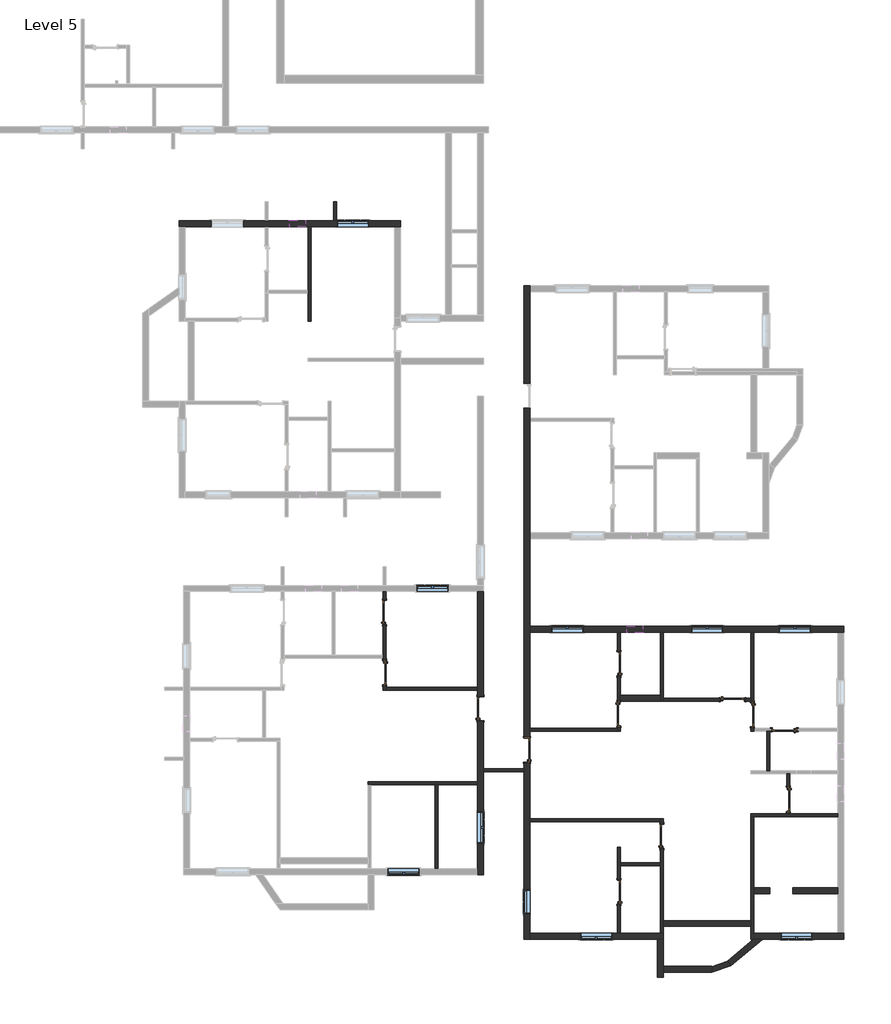
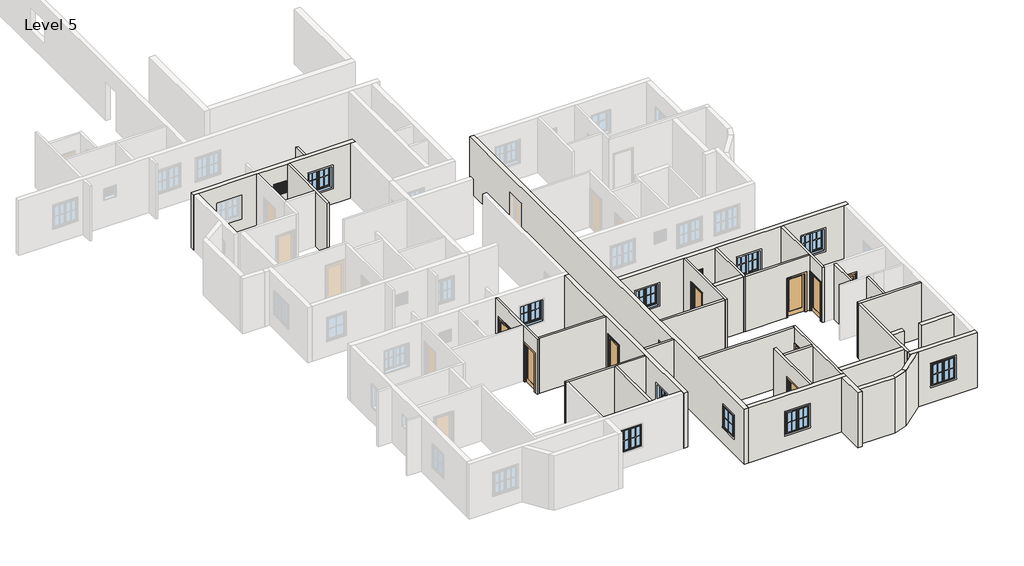
# One storey, part 2 of 7: 34 walls, 12 doors, 12 windows.
"""IFC4 building model written with IfcOpenShell, lengths in millimetres."""

from ifc_helpers import new_model, si_unit, frame, origin, place, context, project, spatial, polyline, circle_curve, outline, extrude, faceted_brep, transform, mapped, element, save
from ifc_brep_helpers import plane_surface, cylinder_surface, revolved_surface, advanced_brep
from components import door_3c6ab76a, door_a3feeac7, door_3b97b8e7, door_868ee8a9, window_272f20d6, window_casement_double_4_x_4_af3140d2, window_f2d8fef0

model = new_model("IFC4")

# Units and contexts
model_context = context("Model", 3, world=origin())
ifc_project = project(units=[si_unit("LENGTHUNIT", "METRE", prefix="MILLI")], contexts=[model_context])

# Site, building, storey
site = spatial("IfcSite", under=ifc_project)
building = spatial("IfcBuilding", under=site)
storey = spatial("IfcBuildingStorey", under=building, Name="Level 5", Elevation=6400.8)

# Doors
placement = place(None, origin())
door_shape = door_3c6ab76a(model_context)
element("IfcDoor", 1, ObjectType="Door-Interior-Single-1_Panel-Wood : 2'6\" x 7' door", at=placement, inside=storey, context=model_context, shape_type="MappedRepresentation", body=[
    mapped(door_shape, transform((13598.2490531, -20317.8247229, 6400.8), x_axis=(1.0, 0.0, 0.0), y_axis=(0.0, 1.0, 0.0), z_axis=(0.0, 0.0, 1.0))),
])
element("IfcDoor", 2, ObjectType="Door-Interior-Single-1_Panel-Wood : 2'6\" x 7' door", at=placement, inside=storey, context=model_context, shape_type="MappedRepresentation", body=[
    mapped(door_shape, transform((15579.4490531, -21467.1747229, 6400.8), x_axis=(-1.0, 0.0, 0.0), y_axis=(0.0, -1.0, 0.0), z_axis=(0.0, 0.0, 1.0))),
])
element("IfcDoor", 3, ObjectType="Door-Interior-Single-1_Panel-Wood : 2'6\" x 7' door", at=placement, inside=storey, context=model_context, shape_type="MappedRepresentation", body=[
    mapped(door_shape, transform((15735.0240531, -24130.9997229, 6400.8), x_axis=(0.0, -1.0, 0.0), y_axis=(1.0, 0.0, 0.0), z_axis=(0.0, 0.0, 1.0))),
])
element("IfcDoor", 4, ObjectType="Door-Interior-Single-1_Panel-Wood : 2'6\" x 7' door", at=placement, inside=storey, context=model_context, shape_type="MappedRepresentation", body=[
    mapped(door_shape, transform((285.4740531, -16985.9538828, 6400.8), x_axis=(0.0, 1.0, 0.0), y_axis=(-1.0, 0.0, 0.0), z_axis=(0.0, 0.0, 1.0))),
])
door_2_shape = door_a3feeac7(model_context)
element("IfcDoor", 5, ObjectType="Door-Interior-Single-1_Panel-Wood : 2'6\" x 7' door", at=placement, inside=storey, context=model_context, shape_type="MappedRepresentation", body=[
    mapped(door_2_shape, transform((9258.0240531, -18949.3997229, 6400.8), x_axis=(0.0, 1.0, 0.0), y_axis=(-1.0, 0.0, 0.0), z_axis=(0.0, 0.0, 1.0))),
])
element("IfcDoor", 6, ObjectType="Door-Interior-Single-1_Panel-Wood : 2'6\" x 7' door", at=placement, inside=storey, context=model_context, shape_type="MappedRepresentation", body=[
    mapped(door_2_shape, transform((9258.0240531, -27674.2997229, 6400.8), x_axis=(0.0, 1.0, 0.0), y_axis=(-1.0, 0.0, 0.0), z_axis=(0.0, 0.0, 1.0))),
])
element("IfcDoor", 7, ObjectType="Door-Interior-Single-1_Panel-Wood : 36\" x 84\"", at=placement, inside=storey, context=model_context, shape_type="MappedRepresentation", body=[
    mapped(door_shape, transform((14363.4240531, -20892.4997229, 6400.8), x_axis=(0.0, -1.0, 0.0), y_axis=(1.0, 0.0, 0.0), z_axis=(0.0, 0.0, 1.0))),
])
element("IfcDoor", 8, ObjectType="Door-Interior-Single-1_Panel-Wood : 36\" x 84\"", at=placement, inside=storey, context=model_context, shape_type="MappedRepresentation", body=[
    mapped(door_shape, transform((10889.9740531, -25540.6997229, 6400.8), x_axis=(0.0, 1.0, 0.0), y_axis=(-1.0, 0.0, 0.0), z_axis=(0.0, 0.0, 1.0))),
])
element("IfcDoor", 9, ObjectType="Door-Interior-Single-1_Panel-Wood : 36\" x 84\"", at=placement, inside=storey, context=model_context, shape_type="MappedRepresentation", body=[
    mapped(door_shape, transform((291.8240531, -19291.0038828, 6400.8), x_axis=(0.0, -1.0, 0.0), y_axis=(1.0, 0.0, 0.0), z_axis=(0.0, 0.0, 1.0))),
])
door_3_shape = door_3b97b8e7(model_context)
element("IfcDoor", 10, ObjectType="Door-Interior-Single-1_Panel-Wood : 36\" x 84\"", at=placement, inside=storey, context=model_context, shape_type="MappedRepresentation", body=[
    mapped(door_3_shape, transform((3962.1240531, -20662.6038828, 6400.8), x_axis=(0.0, 1.0, 0.0), y_axis=(-1.0, 0.0, 0.0), z_axis=(0.0, 0.0, 1.0))),
])
element("IfcDoor", 11, ObjectType="Door-Interior-Single-1_Panel-Wood : 36\" x 84\"", at=placement, inside=storey, context=model_context, shape_type="MappedRepresentation", body=[
    mapped(door_2_shape, transform((9251.6740531, -20863.9247229, 6400.8), x_axis=(0.0, -1.0, 0.0), y_axis=(1.0, 0.0, 0.0), z_axis=(0.0, 0.0, 1.0))),
])
door_4_shape = door_868ee8a9(model_context)
element("IfcDoor", 12, ObjectType="Door-Interior-Single-1_Panel-Wood : 36\" x 84\"", at=placement, inside=storey, context=model_context, shape_type="MappedRepresentation", body=[
    mapped(door_4_shape, transform((5733.7740531, -22245.3540434, 6400.8), x_axis=(0.0, 1.0, 0.0), y_axis=(-1.0, 0.0, 0.0), z_axis=(0.0, 0.0, 1.0))),
])

# Walls
element("IfcWall", 13, ObjectType="4.5\" wall", at=placement, inside=storey, context=model_context, shape_type="Brep", body=[
    faceted_brep([(-2524.4009469, -5860.7538828, 6400.8), (-2524.4009469, -2241.2538828, 6400.8), (-2524.4009469, -2241.2538828, 9448.8), (-2524.4009469, -5860.7538828, 9448.8), (-2638.7009469, -5860.7538828, 6400.8), (-2638.7009469, -5860.7538828, 9448.8), (-2638.7009469, -4793.9538828, 9448.8), (-2638.7009469, -4679.6538828, 9448.8), (-2638.7009469, -2241.2538828, 9448.8), (-2638.7009469, -2241.2538828, 6400.8), (-2638.7009469, -4679.6538828, 6400.8), (-2638.7009469, -4793.9538828, 6400.8)], [[[0, 1, 2, 3]], [[4, 5, 6, 7, 8, 9, 10, 11]], [[1, 0, 4, 11, 10, 9]], [[3, 2, 8, 7, 6, 5]], [[0, 3, 5, 4]], [[2, 1, 9, 8]]]),
])
element("IfcWall", 14, ObjectType="4.5\" wall", at=placement, inside=storey, context=model_context, shape_type="SweptSolid", body=[
    extrude(outline(polyline([(-1533.8009469, -1288.7538828), (-1533.8009469, -2012.6538828), (-1648.1009469, -2012.6538828), (-1648.1009469, -1288.7538828), (-1533.8009469, -1288.7538828)])), frame((0.0, 0.0, 6400.8), z_axis=(0.0, 0.0, 1.0), x_axis=(1.0, 0.0, 0.0)), (0.0, 0.0, 1.0), 3048.0),
])
element("IfcWall", 15, ObjectType="4.5\" wall", at=placement, inside=storey, context=model_context, shape_type="Brep", body=[
    faceted_brep([(345.7990531, -16185.8538828, 9448.8), (345.7990531, -19843.4538828, 9448.8), (345.7990531, -19957.7538828, 9448.8), (345.7990531, -19957.7538828, 6400.8), (345.7990531, -19843.4538828, 6400.8), (345.7990531, -19773.6038828, 6400.8), (345.7990531, -19773.6038828, 8559.8), (345.7990531, -18808.4038828, 8559.8), (345.7990531, -18808.4038828, 6400.8), (345.7990531, -17468.5538828, 6400.8), (345.7990531, -17468.5538828, 8559.8), (345.7990531, -16503.3538828, 8559.8), (345.7990531, -16503.3538828, 6400.8), (345.7990531, -16185.8538828, 6400.8), (231.4990531, -19957.7538828, 9448.8), (231.4990531, -18738.5538828, 9448.8), (231.4990531, -18624.2538828, 9448.8), (231.4990531, -16185.8538828, 9448.8), (231.4990531, -16185.8538828, 6400.8), (231.4990531, -16503.3538828, 6400.8), (231.4990531, -16503.3538828, 8559.8), (231.4990531, -17468.5538828, 8559.8), (231.4990531, -17468.5538828, 6400.8), (231.4990531, -18624.2538828, 6400.8), (231.4990531, -18738.5538828, 6400.8), (231.4990531, -18808.4038828, 6400.8), (231.4990531, -18808.4038828, 8559.8), (231.4990531, -19773.6038828, 8559.8), (231.4990531, -19773.6038828, 6400.8), (231.4990531, -19957.7538828, 6400.8)], [[[0, 1, 2, 3, 4, 5, 6, 7, 8, 9, 10, 11, 12, 13]], [[14, 15, 16, 17, 18, 19, 20, 21, 22, 23, 24, 25, 26, 27, 28, 29]], [[18, 13, 12, 19]], [[3, 29, 28, 5, 4]], [[22, 9, 8, 25, 24, 23]], [[2, 1, 0, 17, 16, 15, 14]], [[0, 13, 18, 17]], [[3, 2, 14, 29]], [[11, 20, 19, 12]], [[20, 11, 10, 21]], [[21, 10, 9, 22]], [[27, 6, 5, 28]], [[6, 27, 26, 7]], [[7, 26, 25, 8]]]),
])
element("IfcWall", 16, ObjectType="4.5\" wall", at=placement, inside=storey, context=model_context, shape_type="SweptSolid", body=[
    extrude(outline(polyline([(3850.9990531, -19957.7538828), (345.7990531, -19957.7538828), (345.7990531, -19843.4538828), (3850.9990531, -19843.4538828), (3850.9990531, -19957.7538828)])), frame((0.0, 0.0, 6400.8), z_axis=(0.0, 0.0, 1.0), x_axis=(1.0, 0.0, 0.0)), (0.0, 0.0, 1.0), 3048.0),
])
element("IfcWall", 17, ObjectType="4.5\" wall", at=placement, inside=storey, context=model_context, shape_type="Brep", body=[
    faceted_brep([(3850.9990531, -23462.9538828, 6400.8), (-340.0009469, -23462.9538828, 6400.8), (-340.0009469, -23462.9538828, 9448.8), (3850.9990531, -23462.9538828, 9448.8), (3850.9990531, -23577.2538828, 6400.8), (3850.9990531, -23577.2538828, 9448.8), (2326.9990531, -23577.2538828, 9448.8), (2212.6990531, -23577.2538828, 9448.8), (-225.7009469, -23577.2538828, 9448.8), (-340.0009469, -23577.2538828, 9448.8), (-340.0009469, -23577.2538828, 6400.8), (-225.7009469, -23577.2538828, 6400.8), (2212.6990531, -23577.2538828, 6400.8), (2326.9990531, -23577.2538828, 6400.8)], [[[0, 1, 2, 3]], [[4, 5, 6, 7, 8, 9, 10, 11, 12, 13]], [[1, 0, 4, 13, 12, 11, 10]], [[3, 2, 9, 8, 7, 6, 5]], [[0, 3, 5, 4]], [[2, 1, 10, 9]]]),
])
element("IfcWall", 18, ObjectType="4.5\" wall", at=placement, inside=storey, context=model_context, shape_type="SweptSolid", body=[
    extrude(outline(polyline([(2326.9990531, -23577.2538828), (2326.9990531, -26777.6538828), (2212.6990531, -26777.6538828), (2212.6990531, -23577.2538828), (2326.9990531, -23577.2538828)])), frame((0.0, 0.0, 6400.8), z_axis=(0.0, 0.0, 1.0), x_axis=(1.0, 0.0, 0.0)), (0.0, 0.0, 1.0), 3048.0),
])
element("IfcWall", 19, ObjectType="4.5\" wall", at=placement, inside=storey, context=model_context, shape_type="Brep", body=[
    faceted_brep([(10835.9990531, -17749.2497229, 6400.8), (10835.9990531, -20149.5497229, 6400.8), (10835.9990531, -20378.1497229, 6400.8), (10835.9990531, -20378.1497229, 9448.8), (10835.9990531, -20149.5497229, 9448.8), (10835.9990531, -17749.2497229, 9448.8), (10950.2990531, -17749.2497229, 6400.8), (10950.2990531, -17749.2497229, 9448.8), (10950.2990531, -20263.8497229, 9448.8), (10950.2990531, -20378.1497229, 9448.8), (10950.2990531, -20378.1497229, 6400.8), (10950.2990531, -20263.8497229, 6400.8)], [[[0, 1, 2, 3, 4, 5]], [[6, 7, 8, 9, 10, 11]], [[2, 1, 0, 6, 11, 10]], [[5, 4, 3, 9, 8, 7]], [[0, 5, 7, 6]], [[3, 2, 10, 9]]]),
])
element("IfcWall", 20, ObjectType="4.5\" wall", at=placement, inside=storey, context=model_context, shape_type="Brep", body=[
    faceted_brep([(9311.9990531, -17749.2497229, 9448.8), (9311.9990531, -20149.5497229, 9448.8), (9311.9990531, -20378.1497229, 9448.8), (9311.9990531, -21521.1497229, 9448.8), (9311.9990531, -21521.1497229, 6400.8), (9311.9990531, -21346.5247229, 6400.8), (9311.9990531, -21346.5247229, 8559.8), (9311.9990531, -20381.3247229, 8559.8), (9311.9990531, -20381.3247229, 6400.8), (9311.9990531, -20378.1497229, 6400.8), (9311.9990531, -20149.5497229, 6400.8), (9311.9990531, -19431.9997229, 6400.8), (9311.9990531, -19431.9997229, 8559.8), (9311.9990531, -18466.7997229, 8559.8), (9311.9990531, -18466.7997229, 6400.8), (9311.9990531, -17749.2497229, 6400.8), (9197.6990531, -21521.1497229, 9448.8), (9197.6990531, -21406.8497229, 9448.8), (9197.6990531, -17749.2497229, 9448.8), (9197.6990531, -17749.2497229, 6400.8), (9197.6990531, -18466.7997229, 6400.8), (9197.6990531, -18466.7997229, 8559.8), (9197.6990531, -19431.9997229, 8559.8), (9197.6990531, -19431.9997229, 6400.8), (9197.6990531, -20381.3247229, 6400.8), (9197.6990531, -20381.3247229, 8559.8), (9197.6990531, -21346.5247229, 8559.8), (9197.6990531, -21346.5247229, 6400.8), (9197.6990531, -21406.8497229, 6400.8), (9197.6990531, -21521.1497229, 6400.8)], [[[0, 1, 2, 3, 4, 5, 6, 7, 8, 9, 10, 11, 12, 13, 14, 15]], [[16, 17, 18, 19, 20, 21, 22, 23, 24, 25, 26, 27, 28, 29]], [[19, 15, 14, 20]], [[4, 29, 28, 27, 5]], [[8, 24, 23, 11, 10, 9]], [[3, 2, 1, 0, 18, 17, 16]], [[0, 15, 19, 18]], [[4, 3, 16, 29]], [[26, 6, 5, 27]], [[6, 26, 25, 7]], [[7, 25, 24, 8]], [[13, 21, 20, 14]], [[21, 13, 12, 22]], [[22, 12, 11, 23]]]),
])
element("IfcWall", 21, ObjectType="4.5\" wall", at=placement, inside=storey, context=model_context, shape_type="SweptSolid", body=[
    extrude(outline(polyline([(5844.8990531, -21406.8497229), (9197.6990531, -21406.8497229), (9197.6990531, -21521.1497229), (5844.8990531, -21521.1497229), (5844.8990531, -21406.8497229)])), frame((0.0, 0.0, 6400.8), z_axis=(0.0, 0.0, 1.0), x_axis=(1.0, 0.0, 0.0)), (0.0, 0.0, 1.0), 3048.0),
])
element("IfcWall", 22, ObjectType="4.5\" wall", at=placement, inside=storey, context=model_context, shape_type="Brep", body=[
    faceted_brep([(14303.0990531, -21521.1497229, 9448.8), (14303.0990531, -20378.1497229, 9448.8), (14303.0990531, -20263.8497229, 9448.8), (14303.0990531, -17749.2497229, 9448.8), (14303.0990531, -17749.2497229, 6400.8), (14303.0990531, -20263.8497229, 6400.8), (14303.0990531, -20378.1497229, 6400.8), (14303.0990531, -20409.8997229, 6400.8), (14303.0990531, -20409.8997229, 8559.8), (14303.0990531, -21375.0997229, 8559.8), (14303.0990531, -21375.0997229, 6400.8), (14303.0990531, -21521.1497229, 6400.8), (14417.3990531, -17749.2497229, 9448.8), (14417.3990531, -21406.8497229, 9448.8), (14417.3990531, -21521.1497229, 9448.8), (14417.3990531, -21521.1497229, 6400.8), (14417.3990531, -21406.8497229, 6400.8), (14417.3990531, -21375.0997229, 6400.8), (14417.3990531, -21375.0997229, 8559.8), (14417.3990531, -20409.8997229, 8559.8), (14417.3990531, -20409.8997229, 6400.8), (14417.3990531, -17749.2497229, 6400.8)], [[[0, 1, 2, 3, 4, 5, 6, 7, 8, 9, 10, 11]], [[12, 13, 14, 15, 16, 17, 18, 19, 20, 21]], [[4, 21, 20, 7, 6, 5]], [[15, 11, 10, 17, 16]], [[3, 2, 1, 0, 14, 13, 12]], [[4, 3, 12, 21]], [[0, 11, 15, 14]], [[9, 18, 17, 10]], [[18, 9, 8, 19]], [[19, 8, 7, 20]]]),
])
element("IfcWall", 23, ObjectType="4.5\" wall", at=placement, inside=storey, context=model_context, shape_type="Brep", body=[
    faceted_brep([(14303.0990531, -24797.7497229, 6400.8), (14417.3990531, -24797.7497229, 6400.8), (17617.7990531, -24797.7497229, 6400.8), (17617.7990531, -24797.7497229, 9448.8), (14417.3990531, -24797.7497229, 9448.8), (14303.0990531, -24797.7497229, 9448.8), (14303.0990531, -24683.4497229, 6400.8), (14303.0990531, -24683.4497229, 9448.8), (15674.6990531, -24683.4497229, 9448.8), (15788.9990531, -24683.4497229, 9448.8), (17617.7990531, -24683.4497229, 9448.8), (17617.7990531, -24683.4497229, 6400.8), (15788.9990531, -24683.4497229, 6400.8), (15674.6990531, -24683.4497229, 6400.8)], [[[0, 1, 2, 3, 4, 5]], [[6, 7, 8, 9, 10, 11, 12, 13]], [[2, 1, 0, 6, 13, 12, 11]], [[5, 4, 3, 10, 9, 8, 7]], [[3, 2, 11, 10]], [[0, 5, 7, 6]]]),
])
element("IfcWall", 24, ObjectType="4.5\" wall", at=placement, inside=storey, context=model_context, shape_type="Brep", body=[
    faceted_brep([(14417.3990531, -29255.4497229, 6400.8), (14417.3990531, -27731.4497229, 6400.8), (14417.3990531, -27502.8497229, 6400.8), (14417.3990531, -24797.7497229, 6400.8), (14417.3990531, -24797.7497229, 9448.8), (14417.3990531, -27502.8497229, 9448.8), (14417.3990531, -27731.4497229, 9448.8), (14417.3990531, -29255.4497229, 9448.8), (14303.0990531, -29255.4497229, 6400.8), (14303.0990531, -29255.4497229, 9448.8), (14303.0990531, -28988.7497229, 9448.8), (14303.0990531, -28760.1497229, 9448.8), (14303.0990531, -24797.7497229, 9448.8), (14303.0990531, -24797.7497229, 6400.8), (14303.0990531, -28760.1497229, 6400.8), (14303.0990531, -28988.7497229, 6400.8)], [[[0, 1, 2, 3, 4, 5, 6, 7]], [[8, 9, 10, 11, 12, 13, 14, 15]], [[3, 2, 1, 0, 8, 15, 14, 13]], [[7, 6, 5, 4, 12, 11, 10, 9]], [[4, 3, 13, 12]], [[0, 7, 9, 8]]]),
])
element("IfcWall", 25, ObjectType="4.5\" wall", at=placement, inside=storey, context=model_context, shape_type="SweptSolid", body=[
    extrude(outline(polyline([(9448.8, 14303.0990531), (9448.8, 10950.2990531), (6400.8, 10950.2990531), (6400.8, 13115.6490531), (8559.8, 13115.6490531), (8559.8, 14080.8490531), (6400.8, 14080.8490531), (6400.8, 14303.0990531), (9448.8, 14303.0990531)])), frame((0.0, -20378.1497229, 0.0), z_axis=(0.0, 1.0, 0.0), x_axis=(0.0, 0.0, 1.0)), (0.0, 0.0, 1.0), 114.3),
])
element("IfcWall", 26, ObjectType="4.5\" wall", at=placement, inside=storey, context=model_context, shape_type="SweptSolid", body=[
    extrude(outline(polyline([(14912.6990531, -23045.1497229), (14912.6990531, -21521.1497229), (15026.9990531, -21521.1497229), (15026.9990531, -23045.1497229), (14912.6990531, -23045.1497229)])), frame((0.0, 0.0, 6400.8), z_axis=(0.0, 0.0, 1.0), x_axis=(1.0, 0.0, 0.0)), (0.0, 0.0, 1.0), 3048.0),
])
element("IfcWall", 27, ObjectType="4.5\" wall", at=placement, inside=storey, context=model_context, shape_type="Brep", body=[
    faceted_brep([(10835.9990531, -29255.4497229, 9448.8), (10835.9990531, -26664.6497229, 9448.8), (10835.9990531, -26550.3497229, 9448.8), (10835.9990531, -24988.2497229, 9448.8), (10835.9990531, -24873.9497229, 9448.8), (10835.9990531, -24873.9497229, 6400.8), (10835.9990531, -24988.2497229, 6400.8), (10835.9990531, -25058.0997229, 6400.8), (10835.9990531, -25058.0997229, 8559.8), (10835.9990531, -26023.2997229, 8559.8), (10835.9990531, -26023.2997229, 6400.8), (10835.9990531, -26550.3497229, 6400.8), (10835.9990531, -26664.6497229, 6400.8), (10835.9990531, -29255.4497229, 6400.8), (10950.2990531, -24873.9497229, 9448.8), (10950.2990531, -28760.1497229, 9448.8), (10950.2990531, -28988.7497229, 9448.8), (10950.2990531, -29255.4497229, 9448.8), (10950.2990531, -29255.4497229, 6400.8), (10950.2990531, -28988.7497229, 6400.8), (10950.2990531, -28760.1497229, 6400.8), (10950.2990531, -26023.2997229, 6400.8), (10950.2990531, -26023.2997229, 8559.8), (10950.2990531, -25058.0997229, 8559.8), (10950.2990531, -25058.0997229, 6400.8), (10950.2990531, -24873.9497229, 6400.8)], [[[0, 1, 2, 3, 4, 5, 6, 7, 8, 9, 10, 11, 12, 13]], [[14, 15, 16, 17, 18, 19, 20, 21, 22, 23, 24, 25]], [[18, 13, 12, 11, 10, 21, 20, 19]], [[5, 25, 24, 7, 6]], [[4, 3, 2, 1, 0, 17, 16, 15, 14]], [[0, 13, 18, 17]], [[5, 4, 14, 25]], [[23, 8, 7, 24]], [[8, 23, 22, 9]], [[9, 22, 21, 10]]]),
])
element("IfcWall", 28, ObjectType="4.5\" wall", at=placement, inside=storey, context=model_context, shape_type="SweptSolid", body=[
    extrude(outline(polyline([(10835.9990531, -24988.2497229), (5844.8990531, -24988.2497229), (5844.8990531, -24873.9497229), (10835.9990531, -24873.9497229), (10835.9990531, -24988.2497229)])), frame((0.0, 0.0, 6400.8), z_axis=(0.0, 0.0, 1.0), x_axis=(1.0, 0.0, 0.0)), (0.0, 0.0, 1.0), 3048.0),
])
element("IfcWall", 29, ObjectType="4.5\" wall", at=placement, inside=storey, context=model_context, shape_type="SweptSolid", body=[
    extrude(outline(polyline([(-24683.4497229, 9448.8), (-23159.4497229, 9448.8), (-23159.4497229, 6400.8), (-23648.3997229, 6400.8), (-23648.3997229, 8559.8), (-24613.5997229, 8559.8), (-24613.5997229, 6400.8), (-24683.4497229, 6400.8), (-24683.4497229, 9448.8)])), frame((15674.6990531, 0.0, 0.0), z_axis=(1.0, 0.0, 0.0), x_axis=(0.0, 1.0, 0.0)), (0.0, 0.0, 1.0), 114.3),
])
element("IfcWall", 30, ObjectType="4.5\" wall", at=placement, inside=storey, context=model_context, shape_type="SweptSolid", body=[
    extrude(outline(polyline([(10835.9990531, -26664.6497229), (9311.9990531, -26664.6497229), (9311.9990531, -26550.3497229), (10835.9990531, -26550.3497229), (10835.9990531, -26664.6497229)])), frame((0.0, 0.0, 6400.8), z_axis=(0.0, 0.0, 1.0), x_axis=(1.0, 0.0, 0.0)), (0.0, 0.0, 1.0), 3048.0),
])
element("IfcWall", 31, ObjectType="4.5\" wall", at=placement, inside=storey, context=model_context, shape_type="Brep", body=[
    faceted_brep([(9311.9990531, -25953.4497229, 6400.8), (9311.9990531, -25953.4497229, 9448.8), (9311.9990531, -26550.3497229, 9448.8), (9311.9990531, -26664.6497229, 9448.8), (9311.9990531, -29255.4497229, 9448.8), (9311.9990531, -29255.4497229, 6400.8), (9311.9990531, -28156.8997229, 6400.8), (9311.9990531, -28156.8997229, 8559.8), (9311.9990531, -27191.6997229, 8559.8), (9311.9990531, -27191.6997229, 6400.8), (9311.9990531, -26664.6497229, 6400.8), (9311.9990531, -26550.3497229, 6400.8), (9197.6990531, -25953.4497229, 9448.8), (9197.6990531, -25953.4497229, 6400.8), (9197.6990531, -27191.6997229, 6400.8), (9197.6990531, -27191.6997229, 8559.8), (9197.6990531, -28156.8997229, 8559.8), (9197.6990531, -28156.8997229, 6400.8), (9197.6990531, -29255.4497229, 6400.8), (9197.6990531, -29255.4497229, 9448.8)], [[[0, 1, 2, 3, 4, 5, 6, 7, 8, 9, 10, 11]], [[12, 13, 14, 15, 16, 17, 18, 19]], [[13, 0, 11, 10, 9, 14]], [[5, 18, 17, 6]], [[1, 0, 13, 12]], [[4, 3, 2, 1, 12, 19]], [[5, 4, 19, 18]], [[8, 15, 14, 9]], [[15, 8, 7, 16]], [[16, 7, 6, 17]]]),
])
element("IfcWall", 32, ObjectType="4.5\" wall", at=placement, inside=storey, context=model_context, shape_type="SweptSolid", body=[
    extrude(outline(polyline([(4079.5990531, -22969.5583639), (5616.2990531, -22969.5583639), (5616.2990531, -23083.8583639), (4079.5990531, -23083.8583639), (4079.5990531, -22969.5583639)])), frame((0.0, 0.0, 6400.8), z_axis=(0.0, 0.0, 1.0), x_axis=(1.0, 0.0, 0.0)), (0.0, 0.0, 1.0), 3048.0),
])
element("IfcWall", 33, ObjectType="9\"", at=placement, inside=storey, context=model_context, shape_type="Brep", body=[
    faceted_brep([(904.5990531, -2012.6538828, 6400.8), (-1533.8009469, -2012.6538828, 6400.8), (-1648.1009469, -2012.6538828, 6400.8), (-4162.7009469, -2012.6538828, 6400.8), (-4277.0009469, -2012.6538828, 6400.8), (-7553.6009469, -2012.6538828, 6400.8), (-7553.6009469, -2012.6538828, 9448.8), (-4277.0009469, -2012.6538828, 9448.8), (-4162.7009469, -2012.6538828, 9448.8), (-1648.1009469, -2012.6538828, 9448.8), (-1533.8009469, -2012.6538828, 9448.8), (904.5990531, -2012.6538828, 9448.8), (-2733.9509469, -2012.6538828, 8534.4), (-3343.5509469, -2012.6538828, 8534.4), (-3343.5509469, -2012.6538828, 7924.8), (-2733.9509469, -2012.6538828, 7924.8), (-5108.8509469, -2012.6538828, 8534.4), (-6328.0509469, -2012.6538828, 8534.4), (-6328.0509469, -2012.6538828, 7315.2), (-5108.8509469, -2012.6538828, 7315.2), (-308.2509469, -2012.6538828, 8534.4), (-1527.4509469, -2012.6538828, 8534.4), (-1527.4509469, -2012.6538828, 7315.2), (-308.2509469, -2012.6538828, 7315.2), (904.5990531, -2241.2538828, 6400.8), (904.5990531, -2241.2538828, 9448.8), (675.9990531, -2241.2538828, 9448.8), (-2524.4009469, -2241.2538828, 9448.8), (-2638.7009469, -2241.2538828, 9448.8), (-4162.7009469, -2241.2538828, 9448.8), (-4277.0009469, -2241.2538828, 9448.8), (-7325.0009469, -2241.2538828, 9448.8), (-7553.6009469, -2241.2538828, 9448.8), (-7553.6009469, -2241.2538828, 6400.8), (-7325.0009469, -2241.2538828, 6400.8), (-4277.0009469, -2241.2538828, 6400.8), (-4162.7009469, -2241.2538828, 6400.8), (-2638.7009469, -2241.2538828, 6400.8), (-2524.4009469, -2241.2538828, 6400.8), (675.9990531, -2241.2538828, 6400.8), (-2733.9509469, -2241.2538828, 8534.4), (-2733.9509469, -2241.2538828, 7924.8), (-3343.5509469, -2241.2538828, 7924.8), (-3343.5509469, -2241.2538828, 8534.4), (-5108.8509469, -2241.2538828, 8534.4), (-5108.8509469, -2241.2538828, 7315.2), (-6328.0509469, -2241.2538828, 7315.2), (-6328.0509469, -2241.2538828, 8534.4), (-308.2509469, -2241.2538828, 8534.4), (-308.2509469, -2241.2538828, 7315.2), (-1527.4509469, -2241.2538828, 7315.2), (-1527.4509469, -2241.2538828, 8534.4)], [[[0, 1, 2, 3, 4, 5, 6, 7, 8, 9, 10, 11], [12, 13, 14, 15], [16, 17, 18, 19], [20, 21, 22, 23]], [[24, 25, 26, 27, 28, 29, 30, 31, 32, 33, 34, 35, 36, 37, 38, 39], [40, 41, 42, 43], [44, 45, 46, 47], [48, 49, 50, 51]], [[5, 4, 3, 2, 1, 0, 24, 39, 38, 37, 36, 35, 34, 33]], [[11, 10, 9, 8, 7, 6, 32, 31, 30, 29, 28, 27, 26, 25]], [[0, 11, 25, 24]], [[6, 5, 33, 32]], [[41, 40, 12, 15]], [[42, 41, 15, 14]], [[43, 42, 14, 13]], [[40, 43, 13, 12]], [[45, 44, 16, 19]], [[46, 45, 19, 18]], [[47, 46, 18, 17]], [[44, 47, 17, 16]], [[49, 48, 20, 23]], [[50, 49, 23, 22]], [[51, 50, 22, 21]], [[48, 51, 21, 20]]]),
])
element("IfcWall", 34, ObjectType="9\"", at=placement, inside=storey, context=model_context, shape_type="Brep", body=[
    faceted_brep([(4079.5990531, -16185.8538828, 9448.8), (4079.5990531, -22969.5583639, 9448.8), (4079.5990531, -23083.8583639, 9448.8), (4079.5990531, -27006.2538828, 9448.8), (4079.5990531, -27006.2538828, 6400.8), (4079.5990531, -23083.8583639, 6400.8), (4079.5990531, -22969.5583639, 6400.8), (4079.5990531, -21145.2038828, 6400.8), (4079.5990531, -21145.2038828, 8559.8), (4079.5990531, -20180.0038828, 8559.8), (4079.5990531, -20180.0038828, 6400.8), (4079.5990531, -16185.8538828, 6400.8), (4079.5990531, -25815.6288828, 8534.4), (4079.5990531, -24596.4288828, 8534.4), (4079.5990531, -24596.4288828, 7315.2), (4079.5990531, -25815.6288828, 7315.2), (3850.9990531, -27006.2538828, 9448.8), (3850.9990531, -26777.6538828, 9448.8), (3850.9990531, -23577.2538828, 9448.8), (3850.9990531, -23462.9538828, 9448.8), (3850.9990531, -19957.7538828, 9448.8), (3850.9990531, -19843.4538828, 9448.8), (3850.9990531, -16185.8538828, 9448.8), (3850.9990531, -16185.8538828, 6400.8), (3850.9990531, -19843.4538828, 6400.8), (3850.9990531, -19957.7538828, 6400.8), (3850.9990531, -20180.0038828, 6400.8), (3850.9990531, -20180.0038828, 8559.8), (3850.9990531, -21145.2038828, 8559.8), (3850.9990531, -21145.2038828, 6400.8), (3850.9990531, -23462.9538828, 6400.8), (3850.9990531, -23577.2538828, 6400.8), (3850.9990531, -26777.6538828, 6400.8), (3850.9990531, -27006.2538828, 6400.8), (3850.9990531, -25815.6288828, 8534.4), (3850.9990531, -25815.6288828, 7315.2), (3850.9990531, -24596.4288828, 7315.2), (3850.9990531, -24596.4288828, 8534.4)], [[[0, 1, 2, 3, 4, 5, 6, 7, 8, 9, 10, 11], [12, 13, 14, 15]], [[16, 17, 18, 19, 20, 21, 22, 23, 24, 25, 26, 27, 28, 29, 30, 31, 32, 33], [34, 35, 36, 37]], [[4, 33, 32, 31, 30, 29, 7, 6, 5]], [[23, 11, 10, 26, 25, 24]], [[3, 2, 1, 0, 22, 21, 20, 19, 18, 17, 16]], [[4, 3, 16, 33]], [[0, 11, 23, 22]], [[9, 27, 26, 10]], [[27, 9, 8, 28]], [[28, 8, 7, 29]], [[35, 34, 12, 15]], [[36, 35, 15, 14]], [[37, 36, 14, 13]], [[34, 37, 13, 12]]]),
])
element("IfcWall", 35, ObjectType="9\"", at=placement, inside=storey, context=model_context, shape_type="Brep", body=[
    faceted_brep([(5844.8990531, -17749.2497229, 6400.8), (9197.6990531, -17749.2497229, 6400.8), (9311.9990531, -17749.2497229, 6400.8), (10835.9990531, -17749.2497229, 6400.8), (10950.2990531, -17749.2497229, 6400.8), (14303.0990531, -17749.2497229, 6400.8), (14417.3990531, -17749.2497229, 6400.8), (17617.7990531, -17749.2497229, 6400.8), (17846.3990531, -17749.2497229, 6400.8), (17846.3990531, -17749.2497229, 9448.8), (17617.7990531, -17749.2497229, 9448.8), (14417.3990531, -17749.2497229, 9448.8), (14303.0990531, -17749.2497229, 9448.8), (10950.2990531, -17749.2497229, 9448.8), (10835.9990531, -17749.2497229, 9448.8), (9311.9990531, -17749.2497229, 9448.8), (9197.6990531, -17749.2497229, 9448.8), (5844.8990531, -17749.2497229, 9448.8), (10169.2490531, -17749.2497229, 8534.4), (10169.2490531, -17749.2497229, 7924.8), (9559.6490531, -17749.2497229, 7924.8), (9559.6490531, -17749.2497229, 8534.4), (7889.5990531, -17749.2497229, 8534.4), (7889.5990531, -17749.2497229, 7315.2), (6670.3990531, -17749.2497229, 7315.2), (6670.3990531, -17749.2497229, 8534.4), (13236.2990531, -17749.2497229, 8534.4), (13236.2990531, -17749.2497229, 7315.2), (12017.0990531, -17749.2497229, 7315.2), (12017.0990531, -17749.2497229, 8534.4), (16595.4490531, -17749.2497229, 8534.4), (16595.4490531, -17749.2497229, 7315.2), (15376.2490531, -17749.2497229, 7315.2), (15376.2490531, -17749.2497229, 8534.4), (5844.8990531, -17520.6497229, 6400.8), (5844.8990531, -17520.6497229, 9448.8), (17846.3990531, -17520.6497229, 9448.8), (17846.3990531, -17520.6497229, 6400.8), (10169.2490531, -17520.6497229, 8534.4), (9559.6490531, -17520.6497229, 8534.4), (9559.6490531, -17520.6497229, 7924.8), (10169.2490531, -17520.6497229, 7924.8), (7889.5990531, -17520.6497229, 8534.4), (6670.3990531, -17520.6497229, 8534.4), (6670.3990531, -17520.6497229, 7315.2), (7889.5990531, -17520.6497229, 7315.2), (13236.2990531, -17520.6497229, 8534.4), (12017.0990531, -17520.6497229, 8534.4), (12017.0990531, -17520.6497229, 7315.2), (13236.2990531, -17520.6497229, 7315.2), (16595.4490531, -17520.6497229, 8534.4), (15376.2490531, -17520.6497229, 8534.4), (15376.2490531, -17520.6497229, 7315.2), (16595.4490531, -17520.6497229, 7315.2)], [[[0, 1, 2, 3, 4, 5, 6, 7, 8, 9, 10, 11, 12, 13, 14, 15, 16, 17], [18, 19, 20, 21], [22, 23, 24, 25], [26, 27, 28, 29], [30, 31, 32, 33]], [[34, 35, 36, 37], [38, 39, 40, 41], [42, 43, 44, 45], [46, 47, 48, 49], [50, 51, 52, 53]], [[8, 7, 6, 5, 4, 3, 2, 1, 0, 34, 37]], [[17, 16, 15, 14, 13, 12, 11, 10, 9, 36, 35]], [[0, 17, 35, 34]], [[9, 8, 37, 36]], [[19, 18, 38, 41]], [[20, 19, 41, 40]], [[21, 20, 40, 39]], [[18, 21, 39, 38]], [[23, 22, 42, 45]], [[24, 23, 45, 44]], [[25, 24, 44, 43]], [[22, 25, 43, 42]], [[27, 26, 46, 49]], [[28, 27, 49, 48]], [[29, 28, 48, 47]], [[26, 29, 47, 46]], [[31, 30, 50, 53]], [[32, 31, 53, 52]], [[33, 32, 52, 51]], [[30, 33, 51, 50]]]),
])
element("IfcWall", 36, ObjectType="9\"", at=placement, inside=storey, context=model_context, shape_type="Brep", body=[
    faceted_brep([(5844.8990531, -4503.1497229, 9448.8), (5844.8990531, -4731.7497229, 9448.8), (5844.8990531, -9557.7497229, 9448.8), (5844.8990531, -9672.0497229, 9448.8), (5844.8990531, -13939.2497229, 9448.8), (5844.8990531, -14167.8497229, 9448.8), (5844.8990531, -17520.6497229, 9448.8), (5844.8990531, -17749.2497229, 9448.8), (5844.8990531, -21406.8497229, 9448.8), (5844.8990531, -21521.1497229, 9448.8), (5844.8990531, -24873.9497229, 9448.8), (5844.8990531, -24988.2497229, 9448.8), (5844.8990531, -29255.4497229, 9448.8), (5844.8990531, -29484.0497229, 9448.8), (5844.8990531, -29484.0497229, 6400.8), (5844.8990531, -29255.4497229, 6400.8), (5844.8990531, -24988.2497229, 6400.8), (5844.8990531, -24873.9497229, 6400.8), (5844.8990531, -22727.9540434, 6400.8), (5844.8990531, -22727.9540434, 8559.8), (5844.8990531, -21762.7540434, 8559.8), (5844.8990531, -21762.7540434, 6400.8), (5844.8990531, -21521.1497229, 6400.8), (5844.8990531, -21406.8497229, 6400.8), (5844.8990531, -17749.2497229, 6400.8), (5844.8990531, -17520.6497229, 6400.8), (5844.8990531, -14167.8497229, 6400.8), (5844.8990531, -13939.2497229, 6400.8), (5844.8990531, -9672.0497229, 6400.8), (5844.8990531, -9557.7497229, 6400.8), (5844.8990531, -9183.0997229, 6400.8), (5844.8990531, -9183.0997229, 8559.8), (5844.8990531, -8217.8997229, 8559.8), (5844.8990531, -8217.8997229, 6400.8), (5844.8990531, -4731.7497229, 6400.8), (5844.8990531, -4503.1497229, 6400.8), (5844.8990531, -27591.7497229, 8534.4), (5844.8990531, -27591.7497229, 7315.2), (5844.8990531, -28506.1497229, 7315.2), (5844.8990531, -28506.1497229, 8534.4), (5616.2990531, -29484.0497229, 9448.8), (5616.2990531, -23083.8583639, 9448.8), (5616.2990531, -22969.5583639, 9448.8), (5616.2990531, -4503.1497229, 9448.8), (5616.2990531, -4503.1497229, 6400.8), (5616.2990531, -8217.8997229, 6400.8), (5616.2990531, -8217.8997229, 8559.8), (5616.2990531, -9183.0997229, 8559.8), (5616.2990531, -9183.0997229, 6400.8), (5616.2990531, -21762.7540434, 6400.8), (5616.2990531, -21762.7540434, 8559.8), (5616.2990531, -22727.9540434, 8559.8), (5616.2990531, -22727.9540434, 6400.8), (5616.2990531, -22969.5583639, 6400.8), (5616.2990531, -23083.8583639, 6400.8), (5616.2990531, -29484.0497229, 6400.8), (5616.2990531, -27591.7497229, 8534.4), (5616.2990531, -28506.1497229, 8534.4), (5616.2990531, -28506.1497229, 7315.2), (5616.2990531, -27591.7497229, 7315.2)], [[[0, 1, 2, 3, 4, 5, 6, 7, 8, 9, 10, 11, 12, 13, 14, 15, 16, 17, 18, 19, 20, 21, 22, 23, 24, 25, 26, 27, 28, 29, 30, 31, 32, 33, 34, 35], [36, 37, 38, 39]], [[40, 41, 42, 43, 44, 45, 46, 47, 48, 49, 50, 51, 52, 53, 54, 55], [56, 57, 58, 59]], [[14, 55, 54, 53, 52, 18, 17, 16, 15]], [[44, 35, 34, 33, 45]], [[48, 30, 29, 28, 27, 26, 25, 24, 23, 22, 21, 49]], [[13, 12, 11, 10, 9, 8, 7, 6, 5, 4, 3, 2, 1, 0, 43, 42, 41, 40]], [[14, 13, 40, 55]], [[0, 35, 44, 43]], [[47, 31, 30, 48]], [[31, 47, 46, 32]], [[32, 46, 45, 33]], [[20, 50, 49, 21]], [[50, 20, 19, 51]], [[51, 19, 18, 52]], [[37, 36, 56, 59]], [[38, 37, 59, 58]], [[39, 38, 58, 57]], [[36, 39, 57, 56]]]),
])
element("IfcWall", 37, ObjectType="9\"", at=placement, inside=storey, context=model_context, shape_type="Brep", body=[
    faceted_brep([(5844.8990531, -29484.0497229, 6400.8), (10721.6990531, -29484.0497229, 6400.8), (10950.2990531, -29484.0497229, 6400.8), (10950.2990531, -29484.0497229, 9448.8), (10721.6990531, -29484.0497229, 9448.8), (5844.8990531, -29484.0497229, 9448.8), (7781.6490531, -29484.0497229, 8534.4), (9000.8490531, -29484.0497229, 8534.4), (9000.8490531, -29484.0497229, 7315.2), (7781.6490531, -29484.0497229, 7315.2), (5844.8990531, -29255.4497229, 6400.8), (5844.8990531, -29255.4497229, 9448.8), (9197.6990531, -29255.4497229, 9448.8), (9311.9990531, -29255.4497229, 9448.8), (10835.9990531, -29255.4497229, 9448.8), (10950.2990531, -29255.4497229, 9448.8), (10950.2990531, -29255.4497229, 6400.8), (10835.9990531, -29255.4497229, 6400.8), (9311.9990531, -29255.4497229, 6400.8), (9197.6990531, -29255.4497229, 6400.8), (7781.6490531, -29255.4497229, 8534.4), (7781.6490531, -29255.4497229, 7315.2), (9000.8490531, -29255.4497229, 7315.2), (9000.8490531, -29255.4497229, 8534.4)], [[[0, 1, 2, 3, 4, 5], [6, 7, 8, 9]], [[10, 11, 12, 13, 14, 15, 16, 17, 18, 19], [20, 21, 22, 23]], [[2, 1, 0, 10, 19, 18, 17, 16]], [[5, 4, 3, 15, 14, 13, 12, 11]], [[0, 5, 11, 10]], [[3, 2, 16, 15]], [[21, 20, 6, 9]], [[22, 21, 9, 8]], [[23, 22, 8, 7]], [[20, 23, 7, 6]]]),
])
element("IfcWall", 38, ObjectType="9\"", at=placement, inside=storey, context=model_context, shape_type="SweptSolid", body=[
    extrude(outline(polyline([(9311.9990531, -20149.5497229), (10835.9990531, -20149.5497229), (10835.9990531, -20378.1497229), (9311.9990531, -20378.1497229), (9311.9990531, -20149.5497229)])), frame((0.0, 0.0, 6400.8), z_axis=(0.0, 0.0, 1.0), x_axis=(1.0, 0.0, 0.0)), (0.0, 0.0, 1.0), 3048.0),
])
element("IfcWall", 39, ObjectType="9\"", at=placement, inside=storey, context=model_context, shape_type="SweptSolid", body=[
    extrude(outline(polyline([(17617.7990531, -27731.4497229), (15901.9350228, -27731.4497229), (15901.9350228, -27502.8497229), (17617.7990531, -27502.8497229), (17617.7990531, -27731.4497229)])), frame((0.0, 0.0, 6400.8), z_axis=(0.0, 0.0, 1.0), x_axis=(1.0, 0.0, 0.0)), (0.0, 0.0, 1.0), 3048.0),
])
element("IfcWall", 40, ObjectType="9\"", at=placement, inside=storey, context=model_context, shape_type="SweptSolid", body=[
    extrude(outline(polyline([(15026.9990531, -27731.4497229), (14417.3990531, -27731.4497229), (14417.3990531, -27502.8497229), (15026.9990531, -27502.8497229), (15026.9990531, -27731.4497229)])), frame((0.0, 0.0, 6400.8), z_axis=(0.0, 0.0, 1.0), x_axis=(1.0, 0.0, 0.0)), (0.0, 0.0, 1.0), 3048.0),
])
element("IfcWall", 41, ObjectType="9\"", at=placement, inside=storey, context=model_context, shape_type="SweptSolid", body=[
    extrude(outline(polyline([(14303.0990531, -28988.7497229), (10950.2990531, -28988.7497229), (10950.2990531, -28760.1497229), (14303.0990531, -28760.1497229), (14303.0990531, -28988.7497229)])), frame((0.0, 0.0, 6400.8), z_axis=(0.0, 0.0, 1.0), x_axis=(1.0, 0.0, 0.0)), (0.0, 0.0, 1.0), 3048.0),
])
element("IfcWall", 42, ObjectType="9\"", at=placement, inside=storey, context=model_context, shape_type="Brep", body=[
    faceted_brep([(14303.0990531, -29484.0497229, 6400.8), (14391.7049387, -29484.0497229, 6400.8), (14750.9761043, -29484.0497229, 6400.8), (17846.3990531, -29484.0497229, 6400.8), (17846.3990531, -29484.0497229, 9448.8), (14750.9761043, -29484.0497229, 9448.8), (14391.7049387, -29484.0497229, 9448.8), (14303.0990531, -29484.0497229, 9448.8), (15436.5740531, -29484.0497229, 8534.4), (16655.7740531, -29484.0497229, 8534.4), (16655.7740531, -29484.0497229, 7315.2), (15436.5740531, -29484.0497229, 7315.2), (14303.0990531, -29255.4497229, 6400.8), (14303.0990531, -29255.4497229, 9448.8), (14417.3990531, -29255.4497229, 9448.8), (17617.7990531, -29255.4497229, 9448.8), (17846.3990531, -29255.4497229, 9448.8), (17846.3990531, -29255.4497229, 6400.8), (17617.7990531, -29255.4497229, 6400.8), (14417.3990531, -29255.4497229, 6400.8), (15436.5740531, -29255.4497229, 8534.4), (15436.5740531, -29255.4497229, 7315.2), (16655.7740531, -29255.4497229, 7315.2), (16655.7740531, -29255.4497229, 8534.4)], [[[0, 1, 2, 3, 4, 5, 6, 7], [8, 9, 10, 11]], [[12, 13, 14, 15, 16, 17, 18, 19], [20, 21, 22, 23]], [[3, 2, 1, 0, 12, 19, 18, 17]], [[7, 6, 5, 4, 16, 15, 14, 13]], [[4, 3, 17, 16]], [[0, 7, 13, 12]], [[21, 20, 8, 11]], [[22, 21, 11, 10]], [[23, 22, 10, 9]], [[20, 23, 9, 8]]]),
])
element("IfcWall", 43, ObjectType="9\"", at=placement, inside=storey, context=model_context, shape_type="Brep", body=[
    faceted_brep([(10950.2990531, -30936.1779934, 6400.8), (10950.2990531, -30741.3497229, 6400.8), (10950.2990531, -30512.7497229, 6400.8), (10950.2990531, -29484.0497229, 6400.8), (10950.2990531, -29484.0497229, 9448.8), (10950.2990531, -30512.7497229, 9448.8), (10950.2990531, -30741.3497229, 9448.8), (10950.2990531, -30936.1779934, 9448.8), (10721.6990531, -30936.1779934, 6400.8), (10721.6990531, -30936.1779934, 9448.8), (10721.6990531, -29484.0497229, 9448.8), (10721.6990531, -29484.0497229, 6400.8)], [[[0, 1, 2, 3, 4, 5, 6, 7]], [[8, 9, 10, 11]], [[3, 2, 1, 0, 8, 11]], [[7, 6, 5, 4, 10, 9]], [[0, 7, 9, 8]], [[4, 3, 11, 10]]]),
])
element("IfcWall", 44, ObjectType="9\"", at=placement, inside=storey, context=model_context, shape_type="Brep", body=[
    faceted_brep([(12809.2934887, -30512.7497229, 6400.8), (10950.2990531, -30512.7497229, 6400.8), (10950.2990531, -30512.7497229, 9448.8), (12809.2934887, -30512.7497229, 9448.8), (12809.2934887, -30741.3497229, 6400.8), (12809.2934887, -30741.3497229, 9448.8), (10950.2990531, -30741.3497229, 9448.8), (10950.2990531, -30741.3497229, 6400.8), (12809.2934887, -30518.3143222, 6400.8), (12809.2934887, -30518.3143222, 9448.8)], [[[0, 1, 2, 3]], [[4, 5, 6, 7]], [[1, 0, 8, 4, 7]], [[3, 2, 6, 5, 9]], [[0, 3, 9, 5, 4, 8]], [[2, 1, 7, 6]]]),
])
element("IfcWall", 45, ObjectType="9\"", at=placement, inside=storey, context=model_context, shape_type="AdvancedBrep", body=[
    advanced_brep(
    [(13391.1154104, -30309.3295271, 9448.8), (12809.2934887, -30518.3143222, 9448.8), (12809.2934887, -30741.3497229, 9448.8), (12809.2934887, -30746.9143222, 9448.8), (13536.5708908, -30485.6833283, 9448.8), (13391.1154104, -30309.3295271, 6400.8), (13536.5708908, -30485.6833283, 6400.8), (12809.2934887, -30746.9143222, 6400.8), (12809.2934887, -30741.3497229, 6400.8), (12809.2934887, -30518.3143222, 6400.8)],
    [
        (0, 1, circle_curve(frame((12809.2934887, -29603.9143222, 9448.8), z_axis=(0.0, 0.0, -1.0), x_axis=(0.0, -1.0, 0.0)), 914.4)),
        (1, 2),
        (2, 3),
        (3, 4, circle_curve(frame((12809.2934887, -29603.9143222, 9448.8), z_axis=(0.0, 0.0, 1.0), x_axis=(0.0, -1.0, 0.0)), 1143.0)),
        (4, 0),
        (5, 6),
        (6, 7, circle_curve(frame((12809.2934887, -29603.9143222, 6400.8), z_axis=(0.0, 0.0, -1.0), x_axis=(0.0, -1.0, 0.0)), 1143.0)),
        (7, 8),
        (8, 9),
        (9, 5, circle_curve(frame((12809.2934887, -29603.9143222, 6400.8), z_axis=(0.0, 0.0, 1.0), x_axis=(0.0, -1.0, 0.0)), 914.4)),
        (0, 5),
        (9, 1),
        (7, 3),
        (6, 4),
    ],
    [
        plane_surface(frame((12809.2934887, -30518.3143222, 9448.8), z_axis=(0.0, 0.0, 1.0), x_axis=(-1.0, 0.0, 0.0))),
        plane_surface(frame((12809.2934887, -30518.3143222, 6400.8), z_axis=(0.0, 0.0, -1.0), x_axis=(1.0, 0.0, 0.0))),
        revolved_surface(polyline([(12809.2934887, -30518.3143222, 6400.8), (12809.2934887, -30518.3143222, 9448.8)]), (12809.2934887, -29603.9143222, 6400.8), (0.0, 0.0, -1.0)),
        plane_surface(frame((12809.2934887, -30518.3143222, 9448.8), z_axis=(-1.0, 0.0, 0.0), x_axis=(0.0, 0.0, -1.0))),
        cylinder_surface(frame((12809.2934887, -29603.9143222, 6400.8), z_axis=(0.0, 0.0, 1.0), x_axis=(0.0, -1.0, 0.0)), 1143.0),
        plane_surface(frame((13536.5708908, -30485.6833283, 9448.8), z_axis=(0.7714514489745903, 0.6362881908970222, 0.0), x_axis=(0.0, 0.0, -1.0))),
    ],
    [
        (0, [[1, 2, 3, 4, 5]]),
        (1, [[6, 7, 8, 9, 10]]),
        (2, [[-1, 11, -10, 12]]),
        (3, [[-3, -2, -12, -9, -8, 13]]),
        (4, [[-4, -13, -7, 14]]),
        (5, [[-5, -14, -6, -11]]),
    ],
),
])
element("IfcWall", 46, ObjectType="9\"", at=placement, inside=storey, context=model_context, shape_type="SweptSolid", body=[
    extrude(outline(polyline([(13391.1154104, -30309.3295271), (14391.7049387, -29484.0497229), (14750.9761043, -29484.0497229), (13536.5708908, -30485.6833283), (13391.1154104, -30309.3295271)])), frame((0.0, 0.0, 6400.8), z_axis=(0.0, 0.0, 1.0), x_axis=(1.0, 0.0, 0.0)), (0.0, 0.0, 1.0), 3048.0),
])

# Windows
window_shape = window_272f20d6(model_context)
element("IfcWindow", 47, ObjectType="Window-Awning-Single : 36\" x 48\"", at=placement, inside=storey, context=model_context, shape_type="MappedRepresentation", body=[
    mapped(window_shape, transform((5730.5990531, -28048.9497229, 6400.8), x_axis=(0.0, 1.0, 0.0), y_axis=(-1.0, 0.0, 0.0), z_axis=(0.0, 0.0, 1.0))),
])
window_casement_double_4_x_4_shape = window_casement_double_4_x_4_af3140d2(model_context)
element("IfcWindow", 48, ObjectType="Window-Casement-Double : 4' x 4'", at=placement, inside=storey, context=model_context, shape_type="MappedRepresentation", body=[
    mapped(window_casement_double_4_x_4_shape, transform((7279.9990531, -17634.9497229, 6400.8), x_axis=(1.0, 0.0, 0.0), y_axis=(0.0, 1.0, 0.0), z_axis=(0.0, 0.0, 1.0))),
])
element("IfcWindow", 49, ObjectType="Window-Casement-Double : 4' x 4'", at=placement, inside=storey, context=model_context, shape_type="MappedRepresentation", body=[
    mapped(window_casement_double_4_x_4_shape, transform((12626.6990531, -17634.9497229, 6400.8), x_axis=(1.0, 0.0, 0.0), y_axis=(0.0, 1.0, 0.0), z_axis=(0.0, 0.0, 1.0))),
])
element("IfcWindow", 50, ObjectType="Window-Casement-Double : 4' x 4'", at=placement, inside=storey, context=model_context, shape_type="MappedRepresentation", body=[
    mapped(window_casement_double_4_x_4_shape, transform((15985.8490531, -17634.9497229, 6400.8), x_axis=(1.0, 0.0, 0.0), y_axis=(0.0, 1.0, 0.0), z_axis=(0.0, 0.0, 1.0))),
])
element("IfcWindow", 51, ObjectType="Window-Casement-Double : 4' x 4'", at=placement, inside=storey, context=model_context, shape_type="MappedRepresentation", body=[
    mapped(window_casement_double_4_x_4_shape, transform((16046.1740531, -29369.7497229, 6400.8), x_axis=(-1.0, 0.0, 0.0), y_axis=(0.0, -1.0, 0.0), z_axis=(0.0, 0.0, 1.0))),
])
element("IfcWindow", 52, ObjectType="Window-Casement-Double : 4' x 4'", at=placement, inside=storey, context=model_context, shape_type="MappedRepresentation", body=[
    mapped(window_casement_double_4_x_4_shape, transform((8391.2490531, -29369.7497229, 6400.8), x_axis=(-1.0, 0.0, 0.0), y_axis=(0.0, -1.0, 0.0), z_axis=(0.0, 0.0, 1.0))),
])
element("IfcWindow", 53, ObjectType="Window-Casement-Double : 4' x 4'", at=placement, inside=storey, context=model_context, shape_type="MappedRepresentation", body=[
    mapped(window_casement_double_4_x_4_shape, transform((3965.2990531, -25206.0288828, 6400.8), x_axis=(0.0, -1.0, 0.0), y_axis=(1.0, 0.0, 0.0), z_axis=(0.0, 0.0, 1.0))),
])
element("IfcWindow", 54, ObjectType="Window-Casement-Double : 4' x 4'", at=placement, inside=storey, context=model_context, shape_type="MappedRepresentation", body=[
    mapped(window_casement_double_4_x_4_shape, transform((1022.0740531, -26891.9538828, 6400.8), x_axis=(-1.0, 0.0, 0.0), y_axis=(0.0, -1.0, 0.0), z_axis=(0.0, 0.0, 1.0))),
])
element("IfcWindow", 55, ObjectType="Window-Casement-Double : 4' x 4'", at=placement, inside=storey, context=model_context, shape_type="MappedRepresentation", body=[
    mapped(window_casement_double_4_x_4_shape, transform((2126.9740531, -16071.5538828, 6400.8), x_axis=(1.0, 0.0, 0.0), y_axis=(0.0, 1.0, 0.0), z_axis=(0.0, 0.0, 1.0))),
])
element("IfcWindow", 56, ObjectType="Window-Casement-Double : 4' x 4'", at=placement, inside=storey, context=model_context, shape_type="MappedRepresentation", body=[
    mapped(window_casement_double_4_x_4_shape, transform((-917.8509469, -2126.9538828, 6400.8), x_axis=(1.0, 0.0, 0.0), y_axis=(0.0, 1.0, 0.0), z_axis=(0.0, 0.0, 1.0))),
])
window_2_shape = window_f2d8fef0(model_context)
element("IfcWindow", 57, ObjectType="Window-Louvers : 24\" x 24\"", at=placement, inside=storey, context=model_context, shape_type="MappedRepresentation", body=[
    mapped(window_2_shape, transform((-3038.7509469, -2133.3038828, 7010.4), x_axis=(-1.0, 0.0, 0.0), y_axis=(0.0, -1.0, 0.0), z_axis=(0.0, 0.0, 1.0))),
])
element("IfcWindow", 58, ObjectType="Window-Louvers : 24\" x 24\"", at=placement, inside=storey, context=model_context, shape_type="MappedRepresentation", body=[
    mapped(window_2_shape, transform((9864.4490531, -17641.2997229, 7010.4), x_axis=(-1.0, 0.0, 0.0), y_axis=(0.0, -1.0, 0.0), z_axis=(0.0, 0.0, 1.0))),
])

save(model, "model.ifc")

# Revit data of these elements
# Type "Door-Interior-Single-1_Panel-Wood : 2'6\" x 7' door"
#   Type Mark = "9"
#   Assembly Code = "C1020300"
#   Analytic Construction = "Wooden"
#   Top Rail = 0' - 4 11/16"
#   Thickness = 0' - 1 3/8"
#   Thermal Resistance (R) = 2.5876 (h·ft²·°F)/BTU
#   Swing Angle [instance default] = 90.00°
#   Stiles = 0' - 4 3/4"
#   Rough Width = 3' - 2"
#   Rough Height = 7' - 1"
#   Height = 7' - 0"
#   Width = 3' - 0"
#   Heat Transfer Coefficient (U) = 0.3865 BTU/(h·ft²·°F)
#   Bottom Rail = 0' - 9 1/8"
#   Trim Material = Cherry
#   Panel Material = Cherry
#   Frame Material = Cherry
#   Door Handle Material = Aluminum
#   Visual Light Transmittance = 0
#   Solar Heat Gain Coefficient = 0
#   Wall Closure = (empty or 0)
#   Function = (empty or 0)
# Type "Door-Interior-Single-1_Panel-Wood : 36\" x 84\""
#   Type Mark = "8"
#   Assembly Code = "C1020300"
#   Analytic Construction = "Wooden"
#   Top Rail = 0' - 4 11/16"
#   Thickness = 0' - 1 3/8"
#   Thermal Resistance (R) = 2.5876 (h·ft²·°F)/BTU
#   Swing Angle [instance default] = 90.00°
#   Stiles = 0' - 4 3/4"
#   Rough Width = 3' - 2"
#   Rough Height = 7' - 1"
#   Height = 7' - 0"
#   Width = 3' - 0"
#   Heat Transfer Coefficient (U) = 0.3865 BTU/(h·ft²·°F)
#   Bottom Rail = 0' - 9 1/8"
#   Trim Material = Cherry
#   Panel Material = Cherry
#   Frame Material = Cherry
#   Door Handle Material = Aluminum
#   Visual Light Transmittance = 0
#   Solar Heat Gain Coefficient = 0
#   Wall Closure = (empty or 0)
#   Function = (empty or 0)
# Type "4.5\" wall"
#   Assembly Code = "B2010"
#   Layers, outside or top first: 0' - 4 1/2" no material (function 1)
# Type "9\""
#   Assembly Code = "B2010"
#   Layers, outside or top first: 0' - 9" no material (function 1)
# Type "Window-Awning-Single : 36\" x 48\""
#   Type Mark = "20"
#   Fire Rating = "0.5h"
#   Assembly Code = "B2020100"
#   Analytic Construction = "Double glazing - domestic"
#   Window Inset [instance default] = 0' - 0"
#   Wall Thickness [instance default] = 0' - 6"
#   Visual Light Transmittance = 0.81
#   Thermal Resistance (R) = 1.8146 (h·ft²·°F)/BTU
#   Solar Heat Gain Coefficient = 0.76
#   Rough Width = 3' - 0 1/2"
#   Rough Height = 4' - 0 1/2"
#   Interior Wall Closure [instance default] = 0' - 2 1/4"
#   Height = 4' - 0"
#   Heat Transfer Coefficient (U) = 0.5511 BTU/(h·ft²·°F)
#   Frame Extension [instance default] = 0' - 0 1/4"
#   Exterior Wall Closure [instance default] = 0' - 1 1/4"
#   Extension Jamb [instance default] = 0' - 2 1/4"
#   Default Sill Height = 3' - 0"
#   Width = 3' - 0"
#   Muntin Visibility = yes
#   Interior Trim Visibility [instance default] = yes
#   Exterior Trim Visibility [instance default] = yes
#   Extension Jamb Visibility [instance default] = yes
#   Muntin Pattern = Muntin Pattern_2x2 : Muntin Pattern_2x2
#   Interior Trim Material = Wood - Stained
#   Interior Trim = Trim-Window-Interior-Flat : Picture Frame
#   Interior Frame Material = Wood - Stained
#   Glass Panel Material = Glass
#   Exterior Trim Material = Clad - White
#   Exterior Trim = Trim-Window-Exterior-Flat : with Sill
#   Exterior Frame Material = Clad - White
#   Wall Closure = (empty or 0)
# Type "Window-Casement-Double : 4' x 4'"
#   Type Mark = "21"
#   Fire Rating = "0.5h"
#   Assembly Code = "B2020100"
#   Analytic Construction = "Double glazing - domestic"
#   Frame Extension [instance default] = 0' - 0 1/4"
#   Window Inset [instance default] = 0' - 0"
#   Wall Thickness [instance default] = 0' - 6"
#   Interior Wall Closure [instance default] = 0' - 2 1/4"
#   Half Width = 2' - 0"
#   Visual Light Transmittance = 0.81
#   Thermal Resistance (R) = 1.8146 (h·ft²·°F)/BTU
#   Solar Heat Gain Coefficient = 0.76
#   Rough Width = 4' - 0 1/2"
#   Rough Height = 4' - 0 1/2"
#   Height = 4' - 0"
#   Heat Transfer Coefficient (U) = 0.5511 BTU/(h·ft²·°F)
#   Exterior Wall Closure [instance default] = 0' - 1 1/4"
#   Extension Jamb [instance default] = 0' - 2 1/4"
#   Default Sill Height = 3' - 0"
#   Width = 4' - 0"
#   Muntin Visibility = yes
#   Interior Trim Visibility [instance default] = yes
#   Exterior Trim Visibility [instance default] = yes
#   Extension Jamb Visibility [instance default] = yes
#   Interior Trim Material = Wood - Stained
#   Muntin Pattern = Muntin Pattern_2x2 : Muntin Pattern_2x2
#   Interior Trim = Trim-Window-Interior-Flat : Picture Frame
#   Interior Frame Material = Wood - Stained
#   Glass Panel Material = Glass
#   Exterior Trim Material = Clad - White
#   Exterior Trim = Trim-Window-Exterior-Flat : with Sill
#   Exterior Frame Material = Clad - White
#   Wall Closure = (empty or 0)
# Type "Window-Louvers : 24\" x 24\""
#   Type Mark = "18"
#   Construction Type Id = "GSP4R"
#   Assembly Code = "B20"
#   Analytic Construction = "1/8 in Pilkington single glazing"
#   Visual Light Transmittance = 0.9
#   Thermal Resistance (R) = 1.53941 (h·ft²·°F)/BTU
#   Solar Heat Gain Coefficient = 0.78
#   Max Height = 1' - 11.74264"
#   Height = 2' - 0"
#   Heat Transfer Coefficient (U) = 0.6496 BTU/(h·ft²·°F)
#   Blade Width [instance default] = 1' - 10 1/2"
#   Blade Vertical Thickness = 0' - 0.35355"
#   Blade Thickness = 0' - 0 1/4"
#   Blade Spacing = 0' - 1 1/2"
#   Blade Height = 0' - 1.85355"
#   Blade Depth = 0' - 3"
#   Blade Angle = 45.00°
#   Default Sill Height = 3' - 0"
#   Trim Projection_Exterior = 0' - 0 1/2"
#   Trim Projection_Interior = 0' - 0 1/2"
#   Trim Width_Exterior = 0' - 1 1/2"
#   Trim Width_Interior = 0' - 1 1/2"
#   Width = 2' - 0"
#   Max Blade Count = 12
#   Define Thermal Properties by = 1
#   Blade Count = 12
#   Frame Material = Birch
#   Louver Material = Birch
#   Trim Exterior Material = Birch
#   Trim Interior Material = Birch
#   Wall Closure = (empty or 0)
# Elements 1, 2, 3, 4, 5, 6 (IfcDoor, "Door-Interior-Single-1_Panel-Wood : 2'6\" x 7' door")
#   Swing Angle = 90.00°
#   Phase Created = New Construction
#   Materials on its faces: "Cherry", "Aluminum"
# Elements 7, 8, 9, 10, 11, 12 (IfcDoor, "Door-Interior-Single-1_Panel-Wood : 36\" x 84\"")
#   Swing Angle = 90.00°
#   Phase Created = New Construction
#   Materials on its faces: "Cherry", "Aluminum"
# Elements 13, 14, 15, 16, 17, 18, 19, 20, 21, 22, 23, 24, 25, 26, 27, 28, 29, 30, 31, 32 (IfcWall, "4.5\" wall")
#   Top Offset = 0' - 0"
#   Base Offset = 0' - 0"
#   wall height = 10' - 0"
#   Phase Created = New Construction
#   Base Constraint = Level 5
#   Top Constraint = Level 6
#   Materials on its faces: "Default Wall"
# Elements 33, 34, 35, 36, 37, 38, 39, 40, 41, 42, 43, 44, 46 (IfcWall, "9\"")
#   Top Offset = 0' - 0"
#   Base Offset = 0' - 0"
#   wall height = 10' - 0"
#   Phase Created = New Construction
#   Base Constraint = Level 5
#   Top Constraint = Level 6
#   Materials on its faces: "Default Wall"
# Element 45 (IfcWall, "9\"")
#   Top Offset = 0' - 0"
#   Base Offset = 0' - 0"
#   Unconnected Height = 20' - 0"
#   wall height = 10' - 0"
#   Phase Created = New Construction
#   Materials on its faces: "Default Wall"
# Element 47 (IfcWindow, "Window-Awning-Single : 36\" x 48\"")
#   Mark = "94"
#   Window Inset = 0' - 0"
#   Interior Wall Closure = 0' - 2 1/4"
#   Frame Extension = 0' - 0 1/4"
#   Exterior Wall Closure = 0' - 1 1/4"
#   Interior Trim Visibility = yes
#   Exterior Trim Visibility = yes
#   Phase Created = New Construction
#   Materials on its faces: "Wood - Stained", "Glass", "Clad - White"
# Element 48 (IfcWindow, "Window-Casement-Double : 4' x 4'")
#   Mark = "111"
#   Window Inset = 0' - 0"
#   Interior Wall Closure = 0' - 2 1/4"
#   Frame Extension = 0' - 0 1/4"
#   Exterior Wall Closure = 0' - 1 1/4"
#   Interior Trim Visibility = yes
#   Exterior Trim Visibility = yes
#   Phase Created = New Construction
